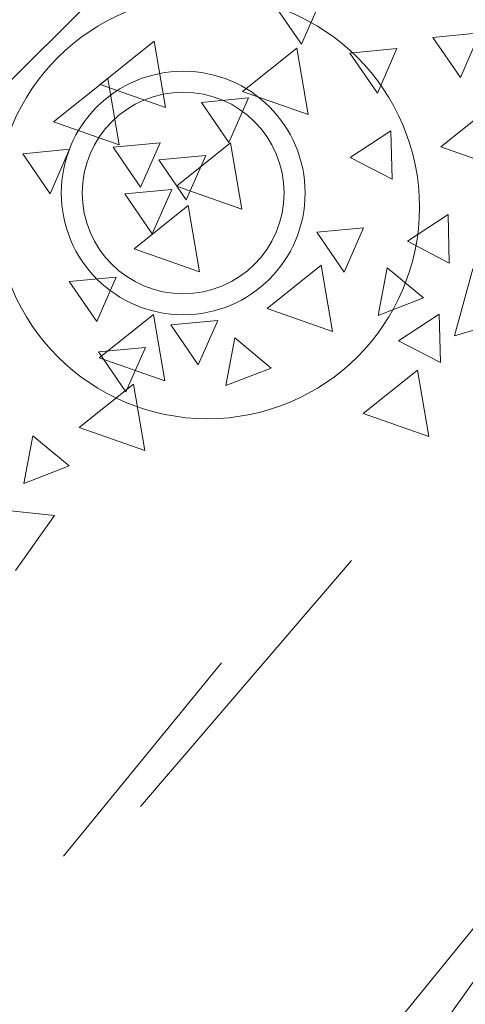
# Model space of a CAD drawing. Units: inches. Extents: x 375 to 1122, y 27 to 1069.
# Tile 104 of 155: x 721 to 731, y 864 to 887. Entities that reach past the tile are written whole.
import ezdxf

# ---------------------------------------------------------------- set-up
doc = ezdxf.new("R2010")
doc.units = ezdxf.units.IN
doc.layers.add('A-ANNO-DIMS', color=2, linetype='Continuous', lineweight=18)
doc.layers.add('Furniture', color=30, linetype='Continuous', lineweight=18)
doc.styles.get("Standard").update_dxf_attribs({"font": 'arial.ttf'})
doc.dimstyles.new('ISO-25', dxfattribs={"dimtxt": 12, "dimasz": 2.5, "dimexe": 1.5, "dimexo": 1.5, "dimtad": 1, "dimdec": 1, "dimlunit": 3, "dimtxsty": 'Standard', "dimblk": 'ARCHTICK', "dimcen": 2.5, "dimadec": 0, "dimazin": 0, "dimtfac": 1, "dimtdec": 1, "dimtmove": 0, "dimatfit": 3, "dimfxl": 1.5, "dimfxlon": 1, "dimarcsym": 0})

# ---------------------------------------------------------------- blocks, each defined once
blk = doc.blocks.new('A$C403C54AD')
for p, q in [((1.46553, 1.19082, -0.0006), (1.47699, 1.15208, -0.0006)), ((1.78922, 1.18993, 0.03663), (1.95298, 1.05694, 0.03663)), ((1.38035, 1.18225, -0.0006), (1.36693, 1.14415, -0.0006)), ((1.83016, 1.1797, 0.03663), (1.90181, 1.12855, 0.03663)), ((1.36693, 1.14415, -0.0006), (1.34169, 1.17565, -0.0006)), ((1.30057, 1.1669, -0.0006), (1.32646, 1.15553, -0.0006)), ((1.30314, 1.13957, -0.0006), (1.30057, 1.1669, -0.0006)), ((1.47699, 1.15208, -0.0006), (1.43807, 1.16281, -0.0006)), ((1.32646, 1.15553, -0.0006), (1.30314, 1.13957, -0.0006)), ((1.40642, 1.1484, -0.0006), (1.43467, 1.14912, -0.0006)), ((1.42197, 1.12477, -0.0006), (1.40642, 1.1484, -0.0006)), ((1.43467, 1.14912, -0.0006), (1.42197, 1.12477, -0.0006)), ((1.46436, 1.14322, -0.0006), (1.49261, 1.14394, -0.0006)), ((1.47991, 1.1196, -0.0006), (1.46436, 1.14322, -0.0006)), ((1.49261, 1.14394, -0.0006), (1.47991, 1.1196, -0.0006)), ((1.49708, 1.13054, -0.0006), (1.53574, 1.13714, -0.0006)), ((1.53574, 1.13714, -0.0006), (1.52232, 1.09903, -0.0006)), ((1.43741, 1.11297, -0.0006), (1.45492, 1.13412, -0.0006)), ((1.45492, 1.13412, -0.0006), (1.46519, 1.10777, -0.0006)), ((1.52232, 1.09903, -0.0006), (1.49708, 1.13054, -0.0006)), ((1.31226, 1.09126, -0.0006), (1.30969, 1.1186, -0.0006)), ((1.30969, 1.1186, -0.0006), (1.33558, 1.10722, -0.0006)), ((1.35757, 1.11509, -0.0006), (1.38582, 1.11581, -0.0006)), ((1.37311, 1.09147, -0.0006), (1.35757, 1.11509, -0.0006)), ((1.38582, 1.11581, -0.0006), (1.37311, 1.09147, -0.0006)), ((1.46519, 1.10777, -0.0006), (1.43741, 1.11297, -0.0006)), ((1.33558, 1.10722, -0.0006), (1.31226, 1.09126, -0.0006)), ((1.41669, 1.07191, -0.0006), (1.41412, 1.09924, -0.0006)), ((1.41412, 1.09924, -0.0006), (1.44001, 1.08787, -0.0006)), ((1.608, 1.0922, -0.0006), (1.75129, 0.96944, -0.0006)), ((1.44001, 1.08787, -0.0006), (1.41669, 1.07191, -0.0006)), ((1.43585, 1.07454, -0.0006), (1.47452, 1.08115, -0.0006)), ((1.47452, 1.08115, -0.0006), (1.4611, 1.04304, -0.0006)), ((1.28124, 1.07437, -0.0006), (1.30713, 1.06299, -0.0006)), ((1.4611, 1.04304, -0.0006), (1.43585, 1.07454, -0.0006)), ((1.30713, 1.06299, -0.0006), (1.28381, 1.04703, -0.0006)), ((1.30948, 1.06033, -0.0006), (1.34815, 1.06694, -0.0006)), ((1.34815, 1.06694, -0.0006), (1.33473, 1.02883, -0.0006)), ((1.33473, 1.02883, -0.0006), (1.30948, 1.06033, -0.0006)), ((1.47832, 1.02428, -0.0006), (1.49583, 1.04543, -0.0006)), ((1.49583, 1.04543, -0.0006), (1.5061, 1.01907, -0.0006)), ((1.34102, 1.00487, -0.0006), (1.33845, 1.03221, -0.0006)), ((1.33845, 1.03221, -0.0006), (1.36435, 1.02083, -0.0006)), ((1.36461, 1.02181, -0.0006), (1.40328, 1.02841, -0.0006)), ((1.40328, 1.02841, -0.0006), (1.38985, 0.99031, -0.0006)), ((1.38985, 0.99031, -0.0006), (1.36461, 1.02181, -0.0006)), ((1.5061, 1.01907, -0.0006), (1.47832, 1.02428, -0.0006)), ((1.36435, 1.02083, -0.0006), (1.34102, 1.00487, -0.0006)), ((1.66765, 1.0166, -0.0006), (1.78023, 0.92452, -0.0006)), ((1.47068, 0.98703, -0.0006), (1.46811, 1.01437, -0.0006)), ((1.46811, 1.01437, -0.0006), (1.494, 1.00299, -0.0006)), ((1.3745, 0.97999, -0.0006), (1.37193, 1.00733, -0.0006)), ((1.37193, 1.00733, -0.0006), (1.39782, 0.99596, -0.0006)), ((1.40106, 0.9971, -0.0006), (1.43972, 1.00371, -0.0006)), ((1.43972, 1.00371, -0.0006), (1.4263, 0.9656, -0.0006)), ((1.494, 1.00299, -0.0006), (1.47068, 0.98703, -0.0006)), ((1.39782, 0.99596, -0.0006), (1.3745, 0.97999, -0.0006)), ((1.4263, 0.9656, -0.0006), (1.40106, 0.9971, -0.0006)), ((1.39427, 0.96028, -0.0006), (1.3917, 0.98762, -0.0006)), ((1.3917, 0.98762, -0.0006), (1.41759, 0.97624, -0.0006)), ((1.30537, 0.97738, -0.0006), (1.34404, 0.98398, -0.0006)), ((1.34404, 0.98398, -0.0006), (1.33062, 0.94587, -0.0006)), ((1.46471, 0.97689, -0.0006), (1.50337, 0.9835, -0.0006)), ((1.50337, 0.9835, -0.0006), (1.48995, 0.94539, -0.0006)), ((1.33062, 0.94587, -0.0006), (1.30537, 0.97738, -0.0006)), ((1.36711, 0.95348, -0.0006), (1.36453, 0.98082, -0.0006)), ((1.36453, 0.98082, -0.0006), (1.39043, 0.96944, -0.0006)), ((1.41759, 0.97624, -0.0006), (1.39427, 0.96028, -0.0006)), ((1.48995, 0.94539, -0.0006), (1.46471, 0.97689, -0.0006)), ((1.48643, 0.9449, -0.0006), (1.48386, 0.97224, -0.0006)), ((1.48386, 0.97224, -0.0006), (1.50975, 0.96086, -0.0006)), ((1.50527, 0.96524, -0.0006), (1.54394, 0.97185, -0.0006)), ((1.54394, 0.97185, -0.0006), (1.53052, 0.93374, -0.0006)), ((1.39043, 0.96944, -0.0006), (1.36711, 0.95348, -0.0006)), ((1.53052, 0.93374, -0.0006), (1.50527, 0.96524, -0.0006)), ((1.50975, 0.96086, -0.0006), (1.48643, 0.9449, -0.0006)), ((1.26636, 0.95578, -0.0006), (1.37894, 0.84325, -0.0006)), ((1.32706, 0.95032, -0.0006), (1.36572, 0.95693, -0.0006)), ((1.36572, 0.95693, -0.0006), (1.3523, 0.91882, -0.0006)), ((1.44544, 0.92794, -0.0006), (1.44286, 0.95528, -0.0006)), ((1.44286, 0.95528, -0.0006), (1.46876, 0.9439, -0.0006)), ((1.3523, 0.91882, -0.0006), (1.32706, 0.95032, -0.0006)), ((1.46876, 0.9439, -0.0006), (1.44544, 0.92794, -0.0006)), ((1.37092, 0.9008, -0.0006), (1.36834, 0.92814, -0.0006)), ((1.36834, 0.92814, -0.0006), (1.39424, 0.91676, -0.0006)), ((1.5354, 0.90675, -0.0006), (1.55291, 0.9279, -0.0006)), ((1.55291, 0.9279, -0.0006), (1.56317, 0.90154, -0.0006)), ((1.57741, 0.87913, -0.0006), (1.58183, 0.91926, -0.0006)), ((1.58183, 0.91926, -0.0006), (1.61385, 0.89659, -0.0006)), ((1.39424, 0.91676, -0.0006), (1.37092, 0.9008, -0.0006)), ((1.56317, 0.90154, -0.0006), (1.5354, 0.90675, -0.0006))]:
    blk.add_line(p, q)
for centre, radius in [((1.40208, 1.00844, -0.0006), 0.12331), ((1.39383, 0.99423, -0.0006), 0.07097), ((1.39383, 0.99423, -0.0006), 0.05876)]:
    blk.add_circle(centre, radius)
blk = doc.blocks.new('_ArchTick')
at = {"color": 0, "linetype": 'ByBlock', "const_width": 0.15}
blk.add_lwpolyline([(-0.5, -0.5), (0.5, 0.5)], dxfattribs=at)
blk = doc.blocks.new('*D85')
at = {"layer": 'A-ANNO-DIMS', "color": 0, "lineweight": -2, "transparency": 16777216}
for p, q in [((401.507, 868.528), (398.507, 868.528)), ((400.007, 814.528), (400.007, 868.528)), ((401.507, 814.528), (398.507, 814.528))]:
    blk.add_line(p, q, dxfattribs=at)
at = {"layer": 'Defpoints', "color": 0, "transparency": 16777216}
for p in [(400.007, 868.528), (845.007, 868.528), (845.007, 814.528)]:
    blk.add_point(p, dxfattribs=at)
at = {"layer": 'A-ANNO-DIMS', "color": 0, "lineweight": -2, "transparency": 16777216, "xscale": 2.5, "yscale": 2.5, "zscale": 2.5}
for p, rotation in [((400.007, 868.528), 90), ((400.007, 814.528), 270)]:
    blk.add_blockref('_ArchTick', p, dxfattribs=dict(at, rotation=rotation))
at = {"layer": 'A-ANNO-DIMS', "color": 0, "transparency": 16777216, "insert": (393.255, 841.528), "char_height": 12, "attachment_point": 5, "rotation": 90}
blk.add_mtext('4\'-6"', dxfattribs=at)
blk = doc.blocks.new('*D88')
at = {"layer": 'A-ANNO-DIMS', "color": 0, "lineweight": -2, "transparency": 16777216}
for p, q in [((731.007, 1052.528), (731.007, 1055.528)), ((854.007, 1052.528), (854.007, 1055.528)), ((731.007, 1054.028), (854.007, 1054.028))]:
    blk.add_line(p, q, dxfattribs=at)
at = {"layer": 'Defpoints', "color": 0, "transparency": 16777216}
for p in [(854.007, 1054.028), (731.007, 502.528), (854.007, 502.528)]:
    blk.add_point(p, dxfattribs=at)
at = {"layer": 'A-ANNO-DIMS', "color": 0, "lineweight": -2, "transparency": 16777216, "xscale": 2.5, "yscale": 2.5, "zscale": 2.5, "rotation": 180}
blk.add_blockref('_ArchTick', (731.007, 1054.028), dxfattribs=at)
at = {"layer": 'A-ANNO-DIMS', "color": 0, "lineweight": -2, "transparency": 16777216, "xscale": 2.5, "yscale": 2.5, "zscale": 2.5}
blk.add_blockref('_ArchTick', (854.007, 1054.028), dxfattribs=at)
at = {"layer": 'A-ANNO-DIMS', "color": 0, "transparency": 16777216, "insert": (792.507, 1060.784), "char_height": 12, "attachment_point": 5}
blk.add_mtext('10\'-3"', dxfattribs=at)
blk = doc.blocks.new('*D91')
at = {"layer": 'A-ANNO-DIMS', "color": 0, "lineweight": -2, "transparency": 16777216}
for p, q in [((728.007, 1052.528), (728.007, 1055.528)), ((788.007, 1052.528), (788.007, 1055.528)), ((728.007, 1054.028), (788.007, 1054.028))]:
    blk.add_line(p, q, dxfattribs=at)
at = {"layer": 'Defpoints', "color": 0, "transparency": 16777216}
for p in [(788.007, 1054.028), (728.007, 774.028), (788.007, 774.028)]:
    blk.add_point(p, dxfattribs=at)
at = {"layer": 'A-ANNO-DIMS', "color": 0, "lineweight": -2, "transparency": 16777216, "xscale": 2.5, "yscale": 2.5, "zscale": 2.5, "rotation": 180}
blk.add_blockref('_ArchTick', (728.007, 1054.028), dxfattribs=at)
at = {"layer": 'A-ANNO-DIMS', "color": 0, "lineweight": -2, "transparency": 16777216, "xscale": 2.5, "yscale": 2.5, "zscale": 2.5}
blk.add_blockref('_ArchTick', (788.007, 1054.028), dxfattribs=at)
at = {"layer": 'A-ANNO-DIMS', "color": 0, "transparency": 16777216, "insert": (758.007, 1060.78), "char_height": 12, "attachment_point": 5}
blk.add_mtext('5\'-0"', dxfattribs=at)

msp = doc.modelspace()

# ---------------------------------------------------------------- block references
at = {"layer": 'Furniture', "xscale": 39.9918517141215, "yscale": 39.9918517141215, "zscale": 39.9918517141215, "rotation": 270}
msp.add_blockref('A$C403C54AD', (684.955, 938.316, 0.024), dxfattribs=at)

# ---------------------------------------------------------------- dimensions: what is measured, and where the dimension line sits
at = {"layer": 'A-ANNO-DIMS'}
for base, p1, p2, picture, middle in [((788.007, 1054.028), (728.007, 774.028), (788.007, 774.028), '*D91', (758.007, 1060.78)), ((854.007, 1054.028), (731.007, 502.528), (854.007, 502.528), '*D88', (792.507, 1060.784))]:
    dim = msp.add_linear_dim(base=base, p1=p1, p2=p2, dimstyle='ISO-25', override={"dimdec": 1, "dimlfac": 1, "dimrnd": 0, "dimzin": 1, "dimdsep": 46, "dimlunit": 4, "dimfrac": 2}, dxfattribs=at)
    dim.commit()
    dim.dimension.update_dxf_attribs({"geometry": picture, "text_midpoint": middle})
dim = msp.add_linear_dim(base=(400.007, 868.528), p1=(845.007, 814.528), p2=(845.007, 868.528), angle=90, dimstyle='ISO-25', override={"dimdec": 1, "dimlfac": 1, "dimrnd": 0, "dimzin": 1, "dimdsep": 46, "dimlunit": 4, "dimfrac": 2}, dxfattribs=at)
dim.commit()
dim.dimension.update_dxf_attribs({"geometry": '*D85', "text_midpoint": (393.255, 841.528)})

doc.saveas('drawing.dxf')
